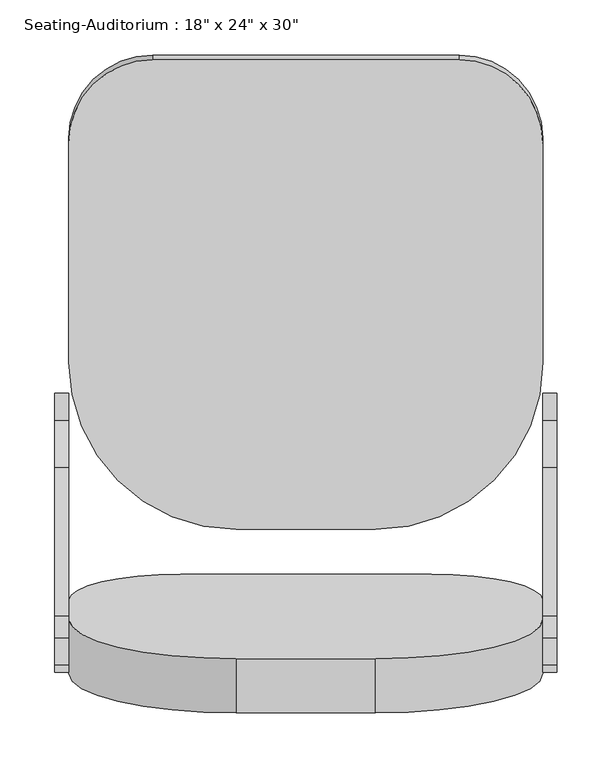
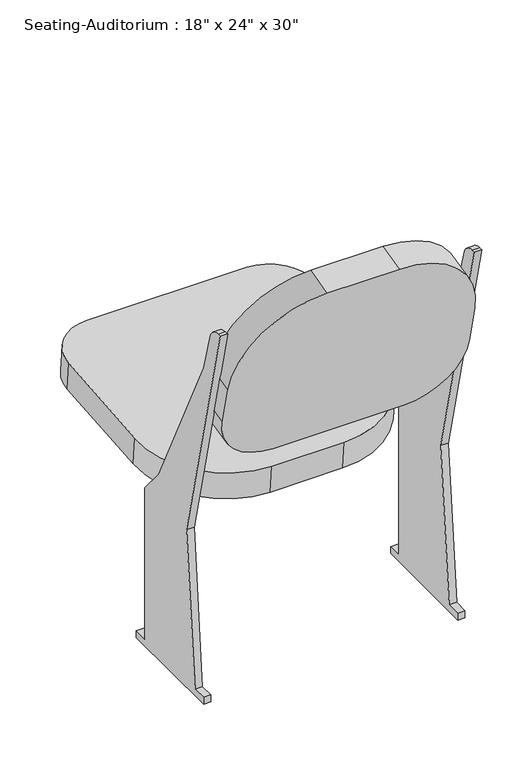
"""IFC4 building model written with IfcOpenShell, lengths in millimetres: furniture geometry."""

from ifc_helpers import new_model, si_unit, point, frame, frame_2d, origin, place, context, project, spatial, polyline, circle_curve, trimmed, segment, composite_curve, outline, extrude, source, transform, mapped, element, save


def furniture_3d1d9cbc(model_context):
    return source(origin(), model_context, "Body", "SweptSolid", [
        extrude(outline(composite_curve([segment(polyline([(0.0, 0.0), (127.0, 0.0)]), True, "CONTINUOUS"), segment(trimmed(circle_curve(frame_2d((127.0, -152.4)), 152.4), [point((127.0, 0.0))], [point((279.4, -152.4))], False, "CARTESIAN"), True, "CONTINUOUS"), segment(polyline([(279.4, -152.4), (279.4, -224.0588601)]), True, "CONTINUOUS"), segment(trimmed(circle_curve(frame_2d((177.8, -224.0588601)), 101.6), [point((279.4, -224.0588601))], [point((177.8, -325.6588601))], False, "CARTESIAN"), True, "CONTINUOUS"), segment(polyline([(177.8, -325.6588601), (-50.8, -325.6588601)]), True, "CONTINUOUS"), segment(trimmed(circle_curve(frame_2d((-50.8, -224.0588601)), 101.6), [point((-50.8, -325.6588601))], [point((-152.4, -224.0588601))], False, "CARTESIAN"), True, "CONTINUOUS"), segment(polyline([(-152.4, -224.0588601), (-152.4, -152.4)]), True, "CONTINUOUS"), segment(trimmed(circle_curve(frame_2d((0.0, -152.4)), 152.4), [point((-152.4, -152.4))], [point((0.0, 0.0))], False, "CARTESIAN"), True, "CONTINUOUS")], self_intersect=False)), frame((224.2278689, -101.3396919, 755.9484479), z_axis=(0.0, 0.9717404775047361, 0.23605178325712217), x_axis=(-1.0, 0.0, 0.0)), (0.0, 0.0, 1.0), 50.8),
        extrude(outline(composite_curve([segment(trimmed(circle_curve(frame_2d((0.0, -76.2)), 76.2), [point((0.0, 0.0))], [point((76.2, -76.2))], False, "CARTESIAN"), True, "CONTINUOUS"), segment(polyline([(76.2, -76.2), (76.2, -276.4123505)]), True, "CONTINUOUS"), segment(trimmed(circle_curve(frame_2d((-76.2, -276.4123505)), 152.4), [point((76.2, -276.4123505))], [point((-76.2, -428.8123506))], False, "CARTESIAN"), True, "CONTINUOUS"), segment(polyline([(-76.2, -428.8123506), (-203.2, -428.8123506)]), True, "CONTINUOUS"), segment(trimmed(circle_curve(frame_2d((-203.2, -276.4123505)), 152.4), [point((-203.2, -428.8123506))], [point((-355.6, -276.4123505))], False, "CARTESIAN"), True, "CONTINUOUS"), segment(polyline([(-355.6, -276.4123505), (-355.6, -76.2)]), True, "CONTINUOUS"), segment(trimmed(circle_curve(frame_2d((-279.4, -76.2)), 76.2), [point((-355.6, -76.2))], [point((-279.4, 0.0))], False, "CARTESIAN"), True, "CONTINUOUS"), segment(polyline([(-279.4, 0.0), (0.0, 0.0)]), True, "CONTINUOUS")], self_intersect=False)), frame((300.4278689, 497.5245173, 321.2380213), z_axis=(0.0, -0.08715574274765496, 0.9961946980917459), x_axis=(1.0, 0.0, 0.0)), (0.0, 0.0, 1.0), 50.8),
        extrude(outline(composite_curve([segment(polyline([(-13.3245902, 0.0), (-13.3245902, 12.7), (12.0754098, 12.7), (37.4754098, 292.1), (-64.1245902, 711.2), (-57.883846, 711.2)]), True, "CONTINUOUS"), segment(trimmed(circle_curve(frame_2d((-57.883846, 685.8)), 25.4), [point((-57.883846, 711.2))], [point((-33.4611378, 692.7779166))], False, "CARTESIAN"), True, "CONTINUOUS"), segment(polyline([(-33.4611378, 692.7779166), (-13.3245902, 622.3), (121.8491486, 342.9), (164.4754098, 292.1), (164.4754098, 12.7), (189.8754098, 12.7), (189.8754098, 0.0), (-13.3245902, 0.0)]), True, "CONTINUOUS")], self_intersect=False)), frame((-67.8721311, 0.0, 0.0), z_axis=(1.0, 0.0, 0.0), x_axis=(0.0, 1.0, 0.0)), (0.0, 0.0, 1.0), 12.7),
        extrude(outline(composite_curve([segment(polyline([(-13.3245902, 12.7), (12.0754098, 12.7), (37.4754098, 292.1), (-64.1245902, 711.2), (-57.883846, 711.2)]), True, "CONTINUOUS"), segment(trimmed(circle_curve(frame_2d((-57.883846, 685.8)), 25.4), [point((-57.883846, 711.2))], [point((-33.4611378, 692.7779166))], False, "CARTESIAN"), True, "CONTINUOUS"), segment(polyline([(-33.4611378, 692.7779166), (-13.3245902, 622.3), (121.8491486, 342.9), (164.4754098, 292.1), (164.4754098, 12.7), (189.8754098, 12.7), (189.8754098, 0.0), (-13.3245902, 0.0), (-13.3245902, 12.7)]), True, "CONTINUOUS")], self_intersect=False)), frame((376.6278689, 0.0, 0.0), z_axis=(1.0, 0.0, 0.0), x_axis=(0.0, 1.0, 0.0)), (0.0, 0.0, 1.0), 12.7),
    ])


if __name__ == "__main__":
    model = new_model("IFC4")
    model_context = context("Model", 3, world=origin())
    ifc_project = project(units=[si_unit("LENGTHUNIT", "METRE", prefix="MILLI")], contexts=[model_context])
    site = spatial("IfcSite", under=ifc_project)
    building = spatial("IfcBuilding", under=site)
    placement = place(None, origin())
    furniture_shape = furniture_3d1d9cbc(model_context)
    element("IfcFurniture", 1, ObjectType="Seating-Auditorium : 18\" x 24\" x 30\"", at=placement, inside=building, context=model_context, shape_type="MappedRepresentation", body=[
        mapped(furniture_shape, transform((0.0, 0.0, 0.0), x_axis=(1.0, 0.0, 0.0), y_axis=(0.0, 1.0, 0.0), z_axis=(0.0, 0.0, 1.0))),
    ])
    save(model, "model.ifc")

# Revit data of these elements
# Type "Seating-Auditorium : 18\" x 24\" x 30\""
#   Assembly Code = "E2020200"
#   Seat Material = Linen, Beige
#   Frame Material = Steel, Paint Finish, Dark Gray, Matte
#   Default Elevation = 0
# Element 1 (IfcFurniture, "Seating-Auditorium : 18\" x 24\" x 30\"")
#   Materials on its faces: "Steel, Paint Finish, Dark Gray, Matte", "Linen, Beige"
# Materials
#   "Linen, Beige": class "Textile", colour RGB 249 239 230, transparency 0, Description = "Linen, beige", Cost = 0
#   "Steel, Paint Finish, Dark Gray, Matte": class "Metal", colour RGB 0 0 0, transparency 0, Description = "Steel, paint finish, dark gray, matte", Cost = 0
